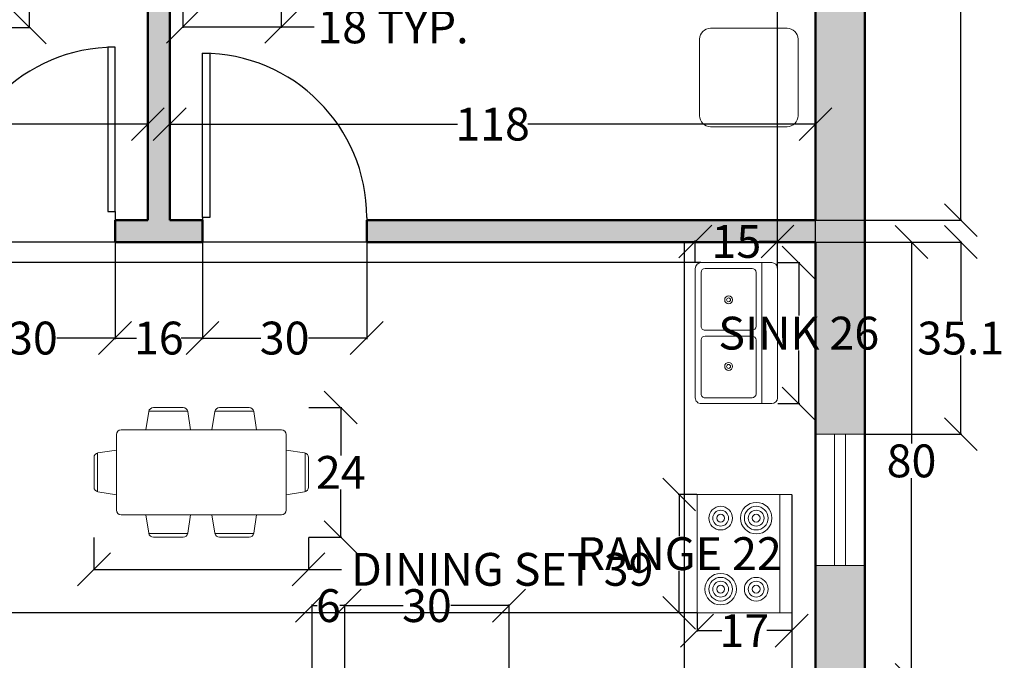
# Model space of a CAD drawing. Units: inches. Extents: x -29 to 284, y -310 to 51.
# Tile 3 of 4: x 105 to 284, y -180 to -63. Entities that reach past the tile are written whole.
import ezdxf

# ---------------------------------------------------------------- set-up
doc = ezdxf.new("R2010")
doc.units = ezdxf.units.IN
doc.header["$MEASUREMENT"] = 0
for name, color, linetype, lineweight in [('A-ANNO-DIMS', 2, 'Continuous', 18), ('A-DOOR', 3, 'Continuous', 25), ('A-EQPM', 8, 'Continuous', 18), ('A-FLOR-CASE', 9, 'Continuous', 25), ('A-FLOR-FIXT', 9, 'Continuous', 18), ('A-FURN', 8, 'Continuous', 18), ('A-GLAZ', 4, 'Continuous', 18), ('A-WALL', 7, 'Continuous', 50)]:
    doc.layers.add(name, color=color, linetype=linetype, lineweight=lineweight)
doc.layers.add('A-WALL-PATT', color=18, linetype='Continuous', lineweight=13, true_color=0x000000)
doc.styles.get("Standard").update_dxf_attribs({"font": 'arial.ttf'})
doc.dimstyles.get("Standard").update_dxf_attribs({"dimtxt": 6, "dimasz": 6, "dimexe": 0.18, "dimexo": 0.0625, "dimgap": 0.09, "dimtad": 0, "dimtih": 1, "dimtoh": 1, "dimdec": 0, "dimzin": 0, "dimdsep": 46, "dimlunit": 4, "dimtxsty": 'Standard', "dimblk": 'OBLIQUE', "dimcen": 0.09, "dimadec": 0, "dimazin": 0, "dimtfac": 1, "dimtdec": 0, "dimtofl": 0, "dimtmove": 0, "dimatfit": 3, "dimldrblk": 'OBLIQUE', "dimfxl": 1, "dimtolj": 1, "dimtzin": 0, "dimarcsym": 0})

# ---------------------------------------------------------------- blocks, each defined once
blk = doc.blocks.new('Range-Oven - 30 in top')
blk.add_line((0, -3), (30, -3))
blk.add_lwpolyline([(0, -24), (0, 0), (30, 0), (30, -24)], close=True)
for centre, radius in [((6, -9), 4), ((6, -9), 3), ((6, -9), 2), ((24, -9), 3), ((24, -9), 2), ((6, -9), 1), ((24, -9), 1), ((24, -18), 4), ((6, -18), 3), ((6, -18), 2), ((6, -18), 1), ((24, -18), 3), ((24, -18), 2), ((24, -18), 1)]:
    blk.add_circle(centre, radius)
blk = doc.blocks.new('Sink-double - 36 in top')
for p, q in [((-18, -4), (18, -4)), ((-0.75, -18.5), (-0.75, -6.5)), ((0.75, -6.5), (0.75, -18.5))]:
    blk.add_line(p, q)
for points in [[(-16.5, 0), (16.5, 0)], [(-18, -19.5), (-18, -1.5)], [(18, -1.5), (18, -19.5)], [(-16.5, -18.5), (-16.5, -6.5)], [(-15.5, -5.5), (-1.75, -5.5)], [(1.75, -5.5), (15.5, -5.5)], [(16.5, -6.5), (16.5, -18.5)], [(-1.75, -19.5), (-15.5, -19.5)], [(15.5, -19.5), (1.75, -19.5)], [(16.5, -21), (-16.5, -21)]]:
    blk.add_lwpolyline(points)
for centre, radius in [((-8.5, -12.5), 1), ((-8.5, -12.5), 0.5), ((8.5, -12.5), 1), ((8.5, -12.5), 0.5)]:
    blk.add_circle(centre, radius)
for centre, radius, start, end in [((-16.5, -1.5), 1.5, 90, 180), ((16.5, -1.5), 1.5, 0, 90), ((-15.5, -6.5), 1, 90, 180), ((-1.75, -6.5), 1, 0, 90), ((1.75, -6.5), 1, 90, 180), ((15.5, -6.5), 1, 0, 90), ((-16.5, -19.5), 1.5, 180, 270), ((-15.5, -18.5), 1, 180, 270), ((-1.75, -18.5), 1, 270, 0), ((1.75, -18.5), 1, 180, 270), ((15.5, -18.5), 1, 270, 0), ((16.5, -19.5), 1.5, 270, 0)]:
    blk.add_arc(centre, radius, start, end)
blk = doc.blocks.new('Dining Set - 36 x 72 in.')
for p, q in [((-22.26, 25.81), (-23.48, 18)), ((-22.23, 26), (-5.76, 26)), ((-20.29, 27.5), (-7.71, 27.5)), ((-4.52, 18), (-5.74, 25.81)), ((5.74, 25.81), (4.52, 18)), ((5.77, 26), (22.24, 26)), ((7.71, 27.5), (20.29, 27.5)), ((23.48, 18), (22.26, 25.81)), ((34, 18), (-34, 18)), ((-36, 16), (-36, -16)), ((36, -16), (36, 16)), ((-43.81, 8.26), (-36, 9.48)), ((43.81, 8.26), (36, 9.48)), ((-45.5, 6.29), (-45.5, -6.29)), ((-44, 8.23), (-44, -8.24)), ((44, 8.23), (44, -8.24)), ((45.5, 6.29), (45.5, -6.29)), ((-36, -9.48), (-43.81, -8.26)), ((36, -9.48), (43.81, -8.26)), ((-34, -18), (34, -18)), ((-22.26, -25.81), (-23.48, -18)), ((-4.52, -18), (-5.74, -25.81)), ((5.74, -25.81), (4.52, -18)), ((23.48, -18), (22.26, -25.81)), ((-22.23, -26), (-5.76, -26)), ((-20.29, -27.5), (-7.71, -27.5)), ((5.77, -26), (22.24, -26)), ((7.71, -27.5), (20.29, -27.5))]:
    blk.add_line(p, q)
for centre, start, end in [((-20.29, 25.5), 90, 171.1198), ((-7.71, 25.5), 8.881, 90), ((7.71, 25.5), 90, 171.1198), ((20.29, 25.5), 8.881, 90), ((-34, 16), 90, 180), ((34, 16), 0, 90), ((-43.5, 6.29), 98.8806, 180), ((43.5, 6.29), 0, 81.1194), ((-43.5, -6.29), 180, 261.1194), ((43.5, -6.29), 278.8806, 0), ((-34, -16), 180, 270), ((34, -16), 270, 0), ((-20.29, -25.5), 188.8802, 270), ((-7.71, -25.5), 270, 351.1191), ((7.71, -25.5), 188.8802, 270), ((20.29, -25.5), 270, 351.1191)]:
    blk.add_arc(centre, 2, start, end)
blk = doc.blocks.new('*U14')
for p, q in [((0, 0), (0, -6)), ((-40, 0), (-40, -6))]:
    blk.add_line(p, q)
blk.add_lwpolyline([(0, 0), (0, 40), (-1.75, 40), (-1.75, 0)], close=True)
blk.add_arc((0, 0), 40, 90, 180)
blk = doc.blocks.new('*U10')
for p, q in [((0, 0), (0, -6)), ((40, 0), (40, -6))]:
    blk.add_line(p, q)
blk.add_lwpolyline([(0, 0), (0, 40), (1.75, 40), (1.75, 0)], close=True)
blk.add_arc((0, 0), 40, 0, 90)
blk = doc.blocks.new('WIN-24IN')
for p, q in [((3.5, 24), (3.5, 0)), ((5.5, 24), (5.5, 0))]:
    blk.add_line(p, q)
for points in [[(0, 24), (9, 24)], [(9, 0), (0, 0)]]:
    blk.add_lwpolyline(points)
blk = doc.blocks.new('NIGHTSTAND-18IN')
blk.add_lwpolyline([(0, 2), (0, 16, -0.414214), (2, 18), (16, 18, -0.414214), (18, 16), (18, 2, -0.414214), (16, 0), (2, 0, -0.414214)], format="xyb", close=True)
blk = doc.blocks.new('_Oblique')
at = {"color": 0, "linetype": 'ByBlock', "lineweight": -2}
blk.add_line((-0.5, -0.5), (0.5, 0.5), dxfattribs=at)
blk = doc.blocks.new('*D26')
at = {"layer": 'A-ANNO-DIMS', "color": 0, "lineweight": -2, "transparency": 16777216}
for p, q in [((94.44, -4.36), (106.56, -4.36)), ((106.38, -4.36), (106.38, -31.2)), ((106.38, -64.36), (106.38, -37.51)), ((94.44, -64.36), (106.56, -64.36))]:
    blk.add_line(p, q, dxfattribs=at)
at = {"layer": 'Defpoints', "color": 0, "transparency": 16777216}
for p in [(94.38, -4.36), (106.38, -4.36), (94.38, -64.36)]:
    blk.add_point(p, dxfattribs=at)
at = {"layer": 'A-ANNO-DIMS', "color": 0, "lineweight": -2, "transparency": 16777216, "xscale": 6, "yscale": 6, "zscale": 6}
for p, rotation in [((106.38, -4.36), 90), ((106.38, -64.36), 270)]:
    blk.add_blockref('_Oblique', p, dxfattribs=dict(at, rotation=rotation))
at = {"layer": 'A-ANNO-DIMS', "color": 0, "transparency": 16777216, "insert": (106.38, -34.36), "char_height": 6, "attachment_point": 5}
blk.add_mtext('\\A1;60 TYP.', dxfattribs=at)
blk = doc.blocks.new('*D32')
at = {"layer": 'A-ANNO-DIMS', "color": 0, "lineweight": -2, "transparency": 16777216}
for p, q in [((134.37, -53.5), (134.37, -64.42)), ((152.37, -53.5), (152.37, -64.42)), ((134.37, -64.24), (152.37, -64.24)), ((152.37, -64.24), (158.37, -64.24))]:
    blk.add_line(p, q, dxfattribs=at)
at = {"layer": 'Defpoints', "color": 0, "transparency": 16777216}
for p in [(134.37, -53.44), (152.37, -53.44), (152.37, -64.24)]:
    blk.add_point(p, dxfattribs=at)
at = {"layer": 'A-ANNO-DIMS', "color": 0, "lineweight": -2, "transparency": 16777216, "xscale": 6, "yscale": 6, "zscale": 6, "rotation": 180}
blk.add_blockref('_Oblique', (134.37, -64.24), dxfattribs=at)
at = {"layer": 'A-ANNO-DIMS', "color": 0, "lineweight": -2, "transparency": 16777216, "xscale": 6, "yscale": 6, "zscale": 6}
blk.add_blockref('_Oblique', (152.37, -64.24), dxfattribs=at)
at = {"layer": 'A-ANNO-DIMS', "color": 0, "transparency": 16777216, "insert": (172.78, -64.24), "char_height": 6, "attachment_point": 5}
blk.add_mtext('\\A1;18 TYP.', dxfattribs=at)
blk = doc.blocks.new('*D33')
at = {"layer": 'A-ANNO-DIMS', "color": 0, "lineweight": -2, "transparency": 16777216}
for p, q in [((228.27, -149.7), (224.9, -149.7)), ((225.08, -149.7), (225.08, -157.32)), ((225.08, -171.33), (225.08, -163.71)), ((228.27, -171.33), (224.9, -171.33))]:
    blk.add_line(p, q, dxfattribs=at)
at = {"layer": 'Defpoints', "color": 0, "transparency": 16777216}
for p in [(228.33, -149.7), (225.08, -171.33), (228.33, -171.33)]:
    blk.add_point(p, dxfattribs=at)
at = {"layer": 'A-ANNO-DIMS', "color": 0, "lineweight": -2, "transparency": 16777216, "xscale": 6, "yscale": 6, "zscale": 6}
for p, rotation in [((225.08, -149.7), 90), ((225.08, -171.33), 270)]:
    blk.add_blockref('_Oblique', p, dxfattribs=dict(at, rotation=rotation))
at = {"layer": 'A-ANNO-DIMS', "color": 0, "transparency": 16777216, "insert": (225.08, -160.51), "char_height": 6, "attachment_point": 5}
blk.add_mtext('\\A1;RANGE 22', dxfattribs=at)
blk = doc.blocks.new('*D34')
at = {"layer": 'A-ANNO-DIMS', "color": 0, "lineweight": -2, "transparency": 16777216}
for p, q in [((228.33, -171.39), (228.33, -174.76)), ((245.64, -171.39), (245.64, -174.76)), ((228.33, -174.58), (232.88, -174.58)), ((245.64, -174.58), (241.09, -174.58))]:
    blk.add_line(p, q, dxfattribs=at)
at = {"layer": 'Defpoints', "color": 0, "transparency": 16777216}
for p in [(228.33, -171.33), (245.64, -171.33), (245.64, -174.58)]:
    blk.add_point(p, dxfattribs=at)
at = {"layer": 'A-ANNO-DIMS', "color": 0, "lineweight": -2, "transparency": 16777216, "xscale": 6, "yscale": 6, "zscale": 6, "rotation": 180}
blk.add_blockref('_Oblique', (228.33, -174.58), dxfattribs=at)
at = {"layer": 'A-ANNO-DIMS', "color": 0, "lineweight": -2, "transparency": 16777216, "xscale": 6, "yscale": 6, "zscale": 6}
blk.add_blockref('_Oblique', (245.64, -174.58), dxfattribs=at)
at = {"layer": 'A-ANNO-DIMS', "color": 0, "transparency": 16777216, "insert": (236.98, -174.58), "char_height": 6, "attachment_point": 5}
blk.add_mtext('\\A1;17', dxfattribs=at)
blk = doc.blocks.new('*D35')
at = {"layer": 'A-ANNO-DIMS', "color": 0, "lineweight": -2, "transparency": 16777216}
for p, q in [((243.12, -107.32), (247.1, -107.32)), ((246.92, -107.32), (246.92, -117.01)), ((246.92, -133.1), (246.92, -123.4)), ((243.12, -133.1), (247.1, -133.1))]:
    blk.add_line(p, q, dxfattribs=at)
at = {"layer": 'Defpoints', "color": 0, "transparency": 16777216}
for p in [(243.05, -107.32), (243.05, -133.1), (246.92, -133.1)]:
    blk.add_point(p, dxfattribs=at)
at = {"layer": 'A-ANNO-DIMS', "color": 0, "lineweight": -2, "transparency": 16777216, "xscale": 6, "yscale": 6, "zscale": 6}
for p, rotation in [((246.92, -107.32), 90), ((246.92, -133.1), 270)]:
    blk.add_blockref('_Oblique', p, dxfattribs=dict(at, rotation=rotation))
at = {"layer": 'A-ANNO-DIMS', "color": 0, "transparency": 16777216, "insert": (246.92, -120.21), "char_height": 6, "attachment_point": 5}
blk.add_mtext('\\A1;SINK 26', dxfattribs=at)
blk = doc.blocks.new('*D36')
at = {"layer": 'A-ANNO-DIMS', "color": 0, "lineweight": -2, "transparency": 16777216}
for p, q in [((228.01, -107.25), (228.01, -103.27)), ((228.01, -103.45), (231.41, -103.45)), ((243.05, -103.45), (239.66, -103.45)), ((243.05, -107.25), (243.05, -103.27))]:
    blk.add_line(p, q, dxfattribs=at)
at = {"layer": 'Defpoints', "color": 0, "transparency": 16777216}
for p in [(243.05, -103.45), (228.01, -107.32), (243.05, -107.32)]:
    blk.add_point(p, dxfattribs=at)
at = {"layer": 'A-ANNO-DIMS', "color": 0, "lineweight": -2, "transparency": 16777216, "xscale": 6, "yscale": 6, "zscale": 6, "rotation": 180}
blk.add_blockref('_Oblique', (228.01, -103.45), dxfattribs=at)
at = {"layer": 'A-ANNO-DIMS', "color": 0, "lineweight": -2, "transparency": 16777216, "xscale": 6, "yscale": 6, "zscale": 6}
blk.add_blockref('_Oblique', (243.05, -103.45), dxfattribs=at)
at = {"layer": 'A-ANNO-DIMS', "color": 0, "transparency": 16777216, "insert": (235.53, -103.45), "char_height": 6, "attachment_point": 5}
blk.add_mtext('\\A1;15', dxfattribs=at)
blk = doc.blocks.new('*D37')
at = {"layer": 'A-ANNO-DIMS', "color": 0, "lineweight": -2, "transparency": 16777216}
for p, q in [((118.14, -157.57), (118.14, -163.56)), ((157.35, -157.57), (157.35, -163.56)), ((118.14, -163.38), (157.35, -163.38)), ((157.35, -163.38), (163.35, -163.38))]:
    blk.add_line(p, q, dxfattribs=at)
at = {"layer": 'Defpoints', "color": 0, "transparency": 16777216}
for p in [(118.14, -157.5), (157.35, -157.5), (157.35, -163.38)]:
    blk.add_point(p, dxfattribs=at)
at = {"layer": 'A-ANNO-DIMS', "color": 0, "lineweight": -2, "transparency": 16777216, "xscale": 6, "yscale": 6, "zscale": 6, "rotation": 180}
blk.add_blockref('_Oblique', (118.14, -163.38), dxfattribs=at)
at = {"layer": 'A-ANNO-DIMS', "color": 0, "lineweight": -2, "transparency": 16777216, "xscale": 6, "yscale": 6, "zscale": 6}
blk.add_blockref('_Oblique', (157.35, -163.38), dxfattribs=at)
at = {"layer": 'A-ANNO-DIMS', "color": 0, "transparency": 16777216, "insert": (192.74, -163.38), "char_height": 6, "attachment_point": 5}
blk.add_mtext('\\A1;DINING SET 39', dxfattribs=at)
blk = doc.blocks.new('*D38')
at = {"layer": 'A-ANNO-DIMS', "color": 0, "lineweight": -2, "transparency": 16777216}
for p, q in [((157.41, -133.81), (163.41, -133.81)), ((163.23, -133.81), (163.23, -142.55)), ((163.23, -157.5), (163.23, -148.76)), ((157.41, -157.5), (163.41, -157.5))]:
    blk.add_line(p, q, dxfattribs=at)
at = {"layer": 'Defpoints', "color": 0, "transparency": 16777216}
for p in [(157.35, -133.81), (163.23, -133.81), (157.35, -157.5)]:
    blk.add_point(p, dxfattribs=at)
at = {"layer": 'A-ANNO-DIMS', "color": 0, "lineweight": -2, "transparency": 16777216, "xscale": 6, "yscale": 6, "zscale": 6}
for p, rotation in [((163.23, -133.81), 90), ((163.23, -157.5), 270)]:
    blk.add_blockref('_Oblique', p, dxfattribs=dict(at, rotation=rotation))
at = {"layer": 'A-ANNO-DIMS', "color": 0, "transparency": 16777216, "insert": (163.23, -145.66), "char_height": 6, "attachment_point": 5}
blk.add_mtext('\\A1;24', dxfattribs=at)
blk = doc.blocks.new('*D51')
at = {"layer": 'A-ANNO-DIMS', "color": 0, "lineweight": -2, "transparency": 16777216}
for p, q in [((250.04, 20.44), (276.71, 20.44)), ((276.53, 20.44), (276.53, -36.41)), ((276.53, -99.56), (276.53, -42.72)), ((250.04, -99.56), (276.71, -99.56))]:
    blk.add_line(p, q, dxfattribs=at)
at = {"layer": 'Defpoints', "color": 0, "transparency": 16777216}
for p in [(249.98, 20.44), (249.98, -99.56), (276.53, -99.56)]:
    blk.add_point(p, dxfattribs=at)
at = {"layer": 'A-ANNO-DIMS', "color": 0, "lineweight": -2, "transparency": 16777216, "xscale": 6, "yscale": 6, "zscale": 6}
for p, rotation in [((276.53, 20.44), 90), ((276.53, -99.56), 270)]:
    blk.add_blockref('_Oblique', p, dxfattribs=dict(at, rotation=rotation))
at = {"layer": 'A-ANNO-DIMS', "color": 0, "transparency": 16777216, "insert": (276.53, -39.56), "char_height": 6, "attachment_point": 5}
blk.add_mtext('\\A1;120', dxfattribs=at)
blk = doc.blocks.new('*D52')
at = {"layer": 'A-ANNO-DIMS', "color": 0, "lineweight": -2, "transparency": 16777216}
for p, q in [((9.98, -99.5), (9.98, -81.83)), ((9.98, -82.01), (62.54, -82.01)), ((127.98, -82.01), (75.42, -82.01)), ((127.98, -99.5), (127.98, -81.83))]:
    blk.add_line(p, q, dxfattribs=at)
at = {"layer": 'Defpoints', "color": 0, "transparency": 16777216}
for p in [(127.98, -82.01), (9.98, -99.56), (127.98, -99.56)]:
    blk.add_point(p, dxfattribs=at)
at = {"layer": 'A-ANNO-DIMS', "color": 0, "lineweight": -2, "transparency": 16777216, "xscale": 6, "yscale": 6, "zscale": 6, "rotation": 180}
blk.add_blockref('_Oblique', (9.98, -82.01), dxfattribs=at)
at = {"layer": 'A-ANNO-DIMS', "color": 0, "lineweight": -2, "transparency": 16777216, "xscale": 6, "yscale": 6, "zscale": 6}
blk.add_blockref('_Oblique', (127.98, -82.01), dxfattribs=at)
at = {"layer": 'A-ANNO-DIMS', "color": 0, "transparency": 16777216, "insert": (68.98, -82.01), "char_height": 6, "attachment_point": 5}
blk.add_mtext('\\A1;118', dxfattribs=at)
blk = doc.blocks.new('*D53')
at = {"layer": 'A-ANNO-DIMS', "color": 0, "lineweight": -2, "transparency": 16777216}
for p, q in [((131.98, -99.5), (131.98, -81.83)), ((131.98, -82.01), (184.54, -82.01)), ((249.98, -82.01), (197.42, -82.01)), ((249.98, -99.5), (249.98, -81.83))]:
    blk.add_line(p, q, dxfattribs=at)
at = {"layer": 'Defpoints', "color": 0, "transparency": 16777216}
for p in [(249.98, -82.01), (131.98, -99.56), (249.98, -99.56)]:
    blk.add_point(p, dxfattribs=at)
at = {"layer": 'A-ANNO-DIMS', "color": 0, "lineweight": -2, "transparency": 16777216, "xscale": 6, "yscale": 6, "zscale": 6, "rotation": 180}
blk.add_blockref('_Oblique', (131.98, -82.01), dxfattribs=at)
at = {"layer": 'A-ANNO-DIMS', "color": 0, "lineweight": -2, "transparency": 16777216, "xscale": 6, "yscale": 6, "zscale": 6}
blk.add_blockref('_Oblique', (249.98, -82.01), dxfattribs=at)
at = {"layer": 'A-ANNO-DIMS', "color": 0, "transparency": 16777216, "insert": (190.98, -82.01), "char_height": 6, "attachment_point": 5}
blk.add_mtext('\\A1;118', dxfattribs=at)
blk = doc.blocks.new('*D55')
at = {"layer": 'A-ANNO-DIMS', "color": 0, "lineweight": -2, "transparency": 16777216}
for p, q in [((91.98, -103.63), (91.98, -121.29)), ((121.98, -103.63), (121.98, -121.29)), ((91.98, -121.11), (102.61, -121.11)), ((121.98, -121.11), (111.36, -121.11))]:
    blk.add_line(p, q, dxfattribs=at)
at = {"layer": 'Defpoints', "color": 0, "transparency": 16777216}
for p in [(91.98, -103.56), (121.98, -103.56), (91.98, -121.11)]:
    blk.add_point(p, dxfattribs=at)
at = {"layer": 'A-ANNO-DIMS', "color": 0, "lineweight": -2, "transparency": 16777216, "xscale": 6, "yscale": 6, "zscale": 6, "rotation": 180}
blk.add_blockref('_Oblique', (91.98, -121.11), dxfattribs=at)
at = {"layer": 'A-ANNO-DIMS', "color": 0, "lineweight": -2, "transparency": 16777216, "xscale": 6, "yscale": 6, "zscale": 6}
blk.add_blockref('_Oblique', (121.98, -121.11), dxfattribs=at)
at = {"layer": 'A-ANNO-DIMS', "color": 0, "transparency": 16777216, "insert": (106.98, -121.11), "char_height": 6, "attachment_point": 5}
blk.add_mtext('\\A1;30', dxfattribs=at)
blk = doc.blocks.new('*D56')
at = {"layer": 'A-ANNO-DIMS', "color": 0, "lineweight": -2, "transparency": 16777216}
for p, q in [((121.98, -103.63), (121.98, -121.29)), ((137.98, -103.63), (137.98, -121.29)), ((121.98, -121.11), (125.88, -121.11)), ((137.98, -121.11), (134.08, -121.11))]:
    blk.add_line(p, q, dxfattribs=at)
at = {"layer": 'Defpoints', "color": 0, "transparency": 16777216}
for p in [(121.98, -103.56), (137.98, -103.56), (121.98, -121.11)]:
    blk.add_point(p, dxfattribs=at)
at = {"layer": 'A-ANNO-DIMS', "color": 0, "lineweight": -2, "transparency": 16777216, "xscale": 6, "yscale": 6, "zscale": 6, "rotation": 180}
blk.add_blockref('_Oblique', (121.98, -121.11), dxfattribs=at)
at = {"layer": 'A-ANNO-DIMS', "color": 0, "lineweight": -2, "transparency": 16777216, "xscale": 6, "yscale": 6, "zscale": 6}
blk.add_blockref('_Oblique', (137.98, -121.11), dxfattribs=at)
at = {"layer": 'A-ANNO-DIMS', "color": 0, "transparency": 16777216, "insert": (129.98, -121.11), "char_height": 6, "attachment_point": 5}
blk.add_mtext('\\A1;16', dxfattribs=at)
blk = doc.blocks.new('*D57')
at = {"layer": 'A-ANNO-DIMS', "color": 0, "lineweight": -2, "transparency": 16777216}
for p, q in [((137.98, -103.63), (137.98, -121.29)), ((167.98, -103.63), (167.98, -121.29)), ((137.98, -121.11), (148.61, -121.11)), ((167.98, -121.11), (157.36, -121.11))]:
    blk.add_line(p, q, dxfattribs=at)
at = {"layer": 'Defpoints', "color": 0, "transparency": 16777216}
for p in [(137.98, -103.56), (167.98, -103.56), (137.98, -121.11)]:
    blk.add_point(p, dxfattribs=at)
at = {"layer": 'A-ANNO-DIMS', "color": 0, "lineweight": -2, "transparency": 16777216, "xscale": 6, "yscale": 6, "zscale": 6, "rotation": 180}
blk.add_blockref('_Oblique', (137.98, -121.11), dxfattribs=at)
at = {"layer": 'A-ANNO-DIMS', "color": 0, "lineweight": -2, "transparency": 16777216, "xscale": 6, "yscale": 6, "zscale": 6}
blk.add_blockref('_Oblique', (167.98, -121.11), dxfattribs=at)
at = {"layer": 'A-ANNO-DIMS', "color": 0, "transparency": 16777216, "insert": (152.98, -121.11), "char_height": 6, "attachment_point": 5}
blk.add_mtext('\\A1;30', dxfattribs=at)
blk = doc.blocks.new('*D64')
at = {"layer": 'A-ANNO-DIMS', "color": 0, "lineweight": -2, "transparency": 16777216}
for p, q in [((250.04, -103.56), (276.71, -103.56)), ((276.53, -103.56), (276.53, -117.96)), ((276.53, -138.66), (276.53, -124.27)), ((259.04, -138.66), (276.71, -138.66))]:
    blk.add_line(p, q, dxfattribs=at)
at = {"layer": 'Defpoints', "color": 0, "transparency": 16777216}
for p in [(249.98, -103.56), (276.53, -103.56), (258.98, -138.66)]:
    blk.add_point(p, dxfattribs=at)
at = {"layer": 'A-ANNO-DIMS', "color": 0, "lineweight": -2, "transparency": 16777216, "xscale": 6, "yscale": 6, "zscale": 6}
for p, rotation in [((276.53, -103.56), 90), ((276.53, -138.66), 270)]:
    blk.add_blockref('_Oblique', p, dxfattribs=dict(at, rotation=rotation))
at = {"layer": 'A-ANNO-DIMS', "color": 0, "transparency": 16777216, "insert": (276.53, -121.11), "char_height": 6, "attachment_point": 5}
blk.add_mtext('\\A1;35.1', dxfattribs=at)
blk = doc.blocks.new('*D65')
at = {"layer": 'A-ANNO-DIMS', "color": 0, "lineweight": -2, "transparency": 16777216}
for p, q in [((250.04, -103.56), (267.71, -103.56)), ((267.53, -103.56), (267.53, -140.41)), ((267.53, -183.56), (267.53, -146.72)), ((250.04, -183.56), (267.71, -183.56))]:
    blk.add_line(p, q, dxfattribs=at)
at = {"layer": 'Defpoints', "color": 0, "transparency": 16777216}
for p in [(249.98, -103.56), (249.98, -183.56), (267.53, -183.56)]:
    blk.add_point(p, dxfattribs=at)
at = {"layer": 'A-ANNO-DIMS', "color": 0, "lineweight": -2, "transparency": 16777216, "xscale": 6, "yscale": 6, "zscale": 6}
for p, rotation in [((267.53, -103.56), 90), ((267.53, -183.56), 270)]:
    blk.add_blockref('_Oblique', p, dxfattribs=dict(at, rotation=rotation))
at = {"layer": 'A-ANNO-DIMS', "color": 0, "transparency": 16777216, "insert": (267.53, -143.56), "char_height": 6, "attachment_point": 5}
blk.add_mtext('\\A1;80', dxfattribs=at)
blk = doc.blocks.new('*D66')
at = {"layer": 'A-ANNO-DIMS', "color": 0, "lineweight": -2, "transparency": 16777216}
for p, q in [((-16.57, -103.56), (-16.57, -97.56)), ((-16.57, -97.56), (-10.57, -97.56)), ((225.92, -103.56), (-16.75, -103.56)), ((-16.57, -107.32), (-16.57, -103.56)), ((229.03, -107.32), (-16.75, -107.32))]:
    blk.add_line(p, q, dxfattribs=at)
at = {"layer": 'Defpoints', "color": 0, "transparency": 16777216}
for p in [(-16.57, -103.56), (225.98, -103.56), (229.09, -107.32)]:
    blk.add_point(p, dxfattribs=at)
at = {"layer": 'A-ANNO-DIMS', "color": 0, "lineweight": -2, "transparency": 16777216, "xscale": 6, "yscale": 6, "zscale": 6}
for p, rotation in [((-16.57, -103.56), 90), ((-16.57, -107.32), 270)]:
    blk.add_blockref('_Oblique', p, dxfattribs=dict(at, rotation=rotation))
at = {"layer": 'A-ANNO-DIMS', "color": 0, "transparency": 16777216, "insert": (-0.39, -97.56), "char_height": 6, "attachment_point": 5}
blk.add_mtext('\\A1;3.752', dxfattribs=at)
blk = doc.blocks.new('*D67')
at = {"layer": 'A-ANNO-DIMS', "color": 0, "lineweight": -2, "transparency": 16777216}
for p, q in [((228.27, -171.33), (-16.75, -171.33)), ((-16.57, -171.33), (-16.57, -174.29)), ((-16.57, -183.56), (-16.57, -180.6)), ((225.92, -183.56), (-16.75, -183.56))]:
    blk.add_line(p, q, dxfattribs=at)
at = {"layer": 'Defpoints', "color": 0, "transparency": 16777216}
for p in [(228.33, -171.33), (-16.57, -183.56), (225.98, -183.56)]:
    blk.add_point(p, dxfattribs=at)
at = {"layer": 'A-ANNO-DIMS', "color": 0, "lineweight": -2, "transparency": 16777216, "xscale": 6, "yscale": 6, "zscale": 6}
for p, rotation in [((-16.57, -171.33), 90), ((-16.57, -183.56), 270)]:
    blk.add_blockref('_Oblique', p, dxfattribs=dict(at, rotation=rotation))
at = {"layer": 'A-ANNO-DIMS', "color": 0, "transparency": 16777216, "insert": (-16.57, -177.45), "char_height": 6, "attachment_point": 5}
blk.add_mtext('\\A1;12.233', dxfattribs=at)
blk = doc.blocks.new('*D68')
at = {"layer": 'A-ANNO-DIMS', "color": 0, "lineweight": -2, "transparency": 16777216}
for p, q in [((243.05, -108.33), (243.05, 47.17)), ((243.05, 46.99), (249.98, 46.99)), ((249.98, -103.5), (249.98, 47.17)), ((249.98, 46.99), (255.98, 46.99))]:
    blk.add_line(p, q, dxfattribs=at)
at = {"layer": 'Defpoints', "color": 0, "transparency": 16777216}
for p in [(249.98, 46.99), (249.98, -103.56), (243.05, -108.39)]:
    blk.add_point(p, dxfattribs=at)
at = {"layer": 'A-ANNO-DIMS', "color": 0, "lineweight": -2, "transparency": 16777216, "xscale": 6, "yscale": 6, "zscale": 6, "rotation": 180}
blk.add_blockref('_Oblique', (243.05, 46.99), dxfattribs=at)
at = {"layer": 'A-ANNO-DIMS', "color": 0, "lineweight": -2, "transparency": 16777216, "xscale": 6, "yscale": 6, "zscale": 6}
blk.add_blockref('_Oblique', (249.98, 46.99), dxfattribs=at)
at = {"layer": 'A-ANNO-DIMS', "color": 0, "transparency": 16777216, "insert": (266.21, 46.99), "char_height": 6, "attachment_point": 5}
blk.add_mtext('\\A1;6.927', dxfattribs=at)
blk = doc.blocks.new('*D69')
at = {"layer": 'A-ANNO-DIMS', "color": 0, "lineweight": -2, "transparency": 16777216}
for p, q in [((249.98, -138.72), (249.98, -306.29)), ((245.64, -149.76), (245.64, -306.29)), ((245.64, -306.11), (249.98, -306.11)), ((249.98, -306.11), (255.98, -306.11))]:
    blk.add_line(p, q, dxfattribs=at)
at = {"layer": 'Defpoints', "color": 0, "transparency": 16777216}
for p in [(249.98, -138.66), (245.64, -149.7), (249.98, -306.11)]:
    blk.add_point(p, dxfattribs=at)
at = {"layer": 'A-ANNO-DIMS', "color": 0, "lineweight": -2, "transparency": 16777216, "xscale": 6, "yscale": 6, "zscale": 6, "rotation": 180}
blk.add_blockref('_Oblique', (245.64, -306.11), dxfattribs=at)
at = {"layer": 'A-ANNO-DIMS', "color": 0, "lineweight": -2, "transparency": 16777216, "xscale": 6, "yscale": 6, "zscale": 6}
blk.add_blockref('_Oblique', (249.98, -306.11), dxfattribs=at)
at = {"layer": 'A-ANNO-DIMS', "color": 0, "transparency": 16777216, "insert": (263.97, -306.11), "char_height": 6, "attachment_point": 5}
blk.add_mtext('\\A1;4.34', dxfattribs=at)
blk = doc.blocks.new('*D73')
at = {"layer": 'A-ANNO-DIMS', "color": 0, "lineweight": -2, "transparency": 16777216}
for p, q in [((157.98, -187.5), (157.98, -169.83)), ((157.98, -170.01), (158.91, -170.01)), ((163.98, -170.01), (163.05, -170.01)), ((163.98, -187.5), (163.98, -169.83))]:
    blk.add_line(p, q, dxfattribs=at)
at = {"layer": 'Defpoints', "color": 0, "transparency": 16777216}
for p in [(163.98, -170.01), (157.98, -187.56), (163.98, -187.56)]:
    blk.add_point(p, dxfattribs=at)
at = {"layer": 'A-ANNO-DIMS', "color": 0, "lineweight": -2, "transparency": 16777216, "xscale": 6, "yscale": 6, "zscale": 6, "rotation": 180}
blk.add_blockref('_Oblique', (157.98, -170.01), dxfattribs=at)
at = {"layer": 'A-ANNO-DIMS', "color": 0, "lineweight": -2, "transparency": 16777216, "xscale": 6, "yscale": 6, "zscale": 6}
blk.add_blockref('_Oblique', (163.98, -170.01), dxfattribs=at)
at = {"layer": 'A-ANNO-DIMS', "color": 0, "transparency": 16777216, "insert": (160.98, -170.01), "char_height": 6, "attachment_point": 5}
blk.add_mtext('\\A1;6', dxfattribs=at)
blk = doc.blocks.new('*D74')
at = {"layer": 'A-ANNO-DIMS', "color": 0, "lineweight": -2, "transparency": 16777216}
for p, q in [((163.98, -187.5), (163.98, -169.83)), ((163.98, -170.01), (174.61, -170.01)), ((193.98, -170.01), (183.36, -170.01)), ((193.98, -187.5), (193.98, -169.83))]:
    blk.add_line(p, q, dxfattribs=at)
at = {"layer": 'Defpoints', "color": 0, "transparency": 16777216}
for p in [(193.98, -170.01), (163.98, -187.56), (193.98, -187.56)]:
    blk.add_point(p, dxfattribs=at)
at = {"layer": 'A-ANNO-DIMS', "color": 0, "lineweight": -2, "transparency": 16777216, "xscale": 6, "yscale": 6, "zscale": 6, "rotation": 180}
blk.add_blockref('_Oblique', (163.98, -170.01), dxfattribs=at)
at = {"layer": 'A-ANNO-DIMS', "color": 0, "lineweight": -2, "transparency": 16777216, "xscale": 6, "yscale": 6, "zscale": 6}
blk.add_blockref('_Oblique', (193.98, -170.01), dxfattribs=at)
at = {"layer": 'A-ANNO-DIMS', "color": 0, "transparency": 16777216, "insert": (178.98, -170.01), "char_height": 6, "attachment_point": 5}
blk.add_mtext('\\A1;30', dxfattribs=at)

msp = doc.modelspace()

# ---------------------------------------------------------------- hatches: boundary and pattern name
at = {"layer": 'A-WALL-PATT'}
h = msp.add_hatch(color=256, dxfattribs=at)
h.dxf.hatch_style = 1
h.paths.add_polyline_path([(172.6409, 20.4365), (172.6409, 29.4365), (82.1984, 29.4365), (82.1984, 20.4365), (127.9809, 20.4365), (127.9809, -99.5635), (121.9809, -99.5635), (121.9809, -103.5635), (127.9809, -103.5635), (137.9809, -103.5635), (137.9809, -99.5635), (131.9809, -99.5635), (131.9809, 20.4365)])
h = msp.add_hatch(color=256, dxfattribs=at)
h.dxf.hatch_style = 1
h.paths.add_polyline_path([(249.9809, 20.4365), (249.9809, -99.5635), (167.9809, -99.5635), (167.9809, -103.5635), (249.9809, -103.5635), (249.9809, -138.6614), (258.9809, -138.6614), (258.9809, 29.4365), (220.6409, 29.4365), (220.6409, 20.4365)])
h = msp.add_hatch(color=256, dxfattribs=at)
h.dxf.hatch_style = 1
h.paths.add_polyline_path([(258.9809, -162.6614), (249.9809, -162.6614), (249.9809, -183.5635), (193.9809, -183.5635), (193.9809, -187.5635), (249.9809, -187.5635), (249.9809, -279.5635), (227.3376, -279.5635), (227.3376, -288.5635), (258.9809, -288.5635)])

# ---------------------------------------------------------------- linework, layer by layer
at = {"layer": 'A-FLOR-CASE'}
msp.add_line((225.9809, -103.5635), (225.9809, -183.5635), dxfattribs=at)
at = {"layer": 'A-WALL'}
for p, q in [((127.9809, -99.5635), (127.9809, 20.4365)), ((131.9809, -99.5635), (131.9809, 20.4365)), ((249.9809, 20.4365), (249.9809, -99.5635)), ((121.9809, -99.5635), (121.9809, -103.5635)), ((121.9809, -99.5635), (127.9809, -99.5635)), ((131.9809, -99.5635), (137.9809, -99.5635)), ((137.9809, -99.5635), (137.9809, -103.5635)), ((167.9809, -99.5635), (167.9809, -103.5635)), ((167.9809, -99.5635), (249.9809, -99.5635)), ((121.9809, -103.5635), (127.9809, -103.5635)), ((127.9809, -103.5635), (137.9809, -103.5635)), ((167.9809, -103.5635), (249.9809, -103.5635)), ((249.9809, -103.5635), (249.9809, -183.5635))]:
    msp.add_line(p, q, dxfattribs=at)
msp.add_lwpolyline([(99.9809, -288.5635), (0.9809, -288.5635), (0.9809, 29.4365), (258.9809, 29.4365), (258.9809, -288.5635), (135.9809, -288.5635)], dxfattribs=at)

# ---------------------------------------------------------------- block references
at = {"layer": 'A-DOOR', "xscale": 0.75, "yscale": 0.75, "zscale": 0.75}
for name, p in [('*U14', (121.9809, -97.9623)), ('*U10', (137.9809, -99.0635))]:
    msp.add_blockref(name, p, dxfattribs=at)
at = {"layer": 'A-EQPM', "xscale": 0.7211102624887981, "yscale": 0.7211102624887981, "zscale": 0.7211102624887981, "rotation": 270}
msp.add_blockref('Range-Oven - 30 in top', (245.6365, -149.6968), dxfattribs=at)
at = {"layer": 'A-FLOR-FIXT', "xscale": 0.7161952055979305, "yscale": 0.7161952055979305, "zscale": 0.7161952055979305, "rotation": 270}
msp.add_blockref('Sink-double - 36 in top', (243.054, -120.2072), dxfattribs=at)
at = {"layer": 'A-FURN', "rotation": 180}
msp.add_blockref('NIGHTSTAND-18IN', (246.7929, -64.4778), dxfattribs=at)
at = {"layer": 'A-FURN', "xscale": 0.430826044735534, "yscale": 0.430826044735534, "zscale": 0.430826044735534}
msp.add_blockref('Dining Set - 36 x 72 in.', (137.7445, -145.6565), dxfattribs=at)
at = {"layer": 'A-GLAZ'}
msp.add_blockref('WIN-24IN', (249.981, -162.661), dxfattribs=at)

# ---------------------------------------------------------------- dimensions: what is measured, and where the dimension line sits
at = {"layer": 'A-ANNO-DIMS'}
for base, p1, p2, override, picture, middle in [((249.9809, 46.9865), (243.054, -108.39), (249.9809, -103.5635), {"dimdec": 3, "dimlfac": 1, "dimrnd": 0, "dimzin": 0, "dimdsep": 46, "dimlunit": 2}, '*D68', (266.2108, 46.9865)), ((127.9809, -82.0135), (9.9809, -99.5635), (127.9809, -99.5635), {"dimdec": 0, "dimlfac": 1, "dimrnd": 0, "dimzin": 0, "dimdsep": 46, "dimlunit": 2}, '*D52', (68.9809, -82.0135)), ((249.9809, -82.0135), (131.9809, -99.5635), (249.9809, -99.5635), {"dimdec": 0, "dimlfac": 1, "dimrnd": 0, "dimzin": 0, "dimdsep": 46, "dimlunit": 2}, '*D53', (190.9809, -82.0135)), ((243.054, -103.4482), (228.0139, -107.3157), (243.054, -107.3157), {"dimdec": 0, "dimlfac": 1, "dimrnd": 0, "dimzin": 0, "dimdsep": 46, "dimlunit": 2}, '*D36', (235.5339, -103.4482)), ((249.9809, -306.1135), (245.6365, -149.6968), (249.9809, -138.6614), {"dimdec": 2, "dimlfac": 1, "dimrnd": 0, "dimzin": 0, "dimdsep": 46, "dimlunit": 2}, '*D69', (263.972, -306.1135)), ((163.9809, -170.0135), (157.9809, -187.5635), (163.9809, -187.5635), {"dimdec": 0, "dimlfac": 1, "dimrnd": 0, "dimzin": 0, "dimdsep": 46, "dimlunit": 2}, '*D73', (160.9809, -170.0135)), ((193.9809, -170.0135), (163.9809, -187.5635), (193.9809, -187.5635), {"dimdec": 0, "dimlfac": 1, "dimrnd": 0, "dimzin": 0, "dimdsep": 46, "dimlunit": 2}, '*D74', (178.9809, -170.0135)), ((245.6365, -174.5751), (228.3299, -171.3301), (245.6365, -171.3301), {"dimdec": 0, "dimlfac": 1, "dimrnd": 0, "dimzin": 0, "dimdsep": 46, "dimlunit": 2}, '*D34', (236.9832, -174.5751))]:
    dim = msp.add_linear_dim(base=base, p1=p1, p2=p2, dimstyle='Standard', override=override, dxfattribs=at)
    dim.commit()
    dim.dimension.update_dxf_attribs({"geometry": picture, "text_midpoint": middle})
for base, p1, p2, angle, override, picture, middle in [((276.5309, -99.5635), (249.9809, 20.4365), (249.9809, -99.5635), 90, {"dimdec": 0, "dimlfac": 1, "dimrnd": 0, "dimzin": 0, "dimdsep": 46, "dimlunit": 2}, '*D51', (276.5309, -39.5635)), ((-16.5691, -103.5635), (229.0882, -107.3157), (225.9809, -103.5635), 90, {"dimdec": 3, "dimlfac": 1, "dimrnd": 0, "dimzin": 0, "dimdsep": 46, "dimlunit": 2}, '*D66', (-0.3883, -97.5635)), ((276.5309, -103.5635), (258.9809, -138.6614), (249.9809, -103.5635), 90, {"dimdec": 1, "dimlfac": 1, "dimrnd": 0, "dimzin": 0, "dimdsep": 46, "dimlunit": 2}, '*D64', (276.5309, -121.1124)), ((267.5309, -183.5635), (249.9809, -103.5635), (249.9809, -183.5635), 270, {"dimdec": 0, "dimlfac": 1, "dimrnd": 0, "dimzin": 0, "dimdsep": 46, "dimlunit": 2}, '*D65', (267.5309, -143.5635)), ((91.9809, -121.1135), (121.9809, -103.5635), (91.9809, -103.5635), 180, {"dimdec": 0, "dimlfac": 1, "dimrnd": 0, "dimzin": 0, "dimdsep": 46, "dimlunit": 2}, '*D55', (106.9809, -121.1135)), ((121.9809, -121.1135), (137.9809, -103.5635), (121.9809, -103.5635), 180, {"dimdec": 0, "dimlfac": 1, "dimrnd": 0, "dimzin": 0, "dimdsep": 46, "dimlunit": 2}, '*D56', (129.9809, -121.1135)), ((137.9809, -121.1135), (167.9809, -103.5635), (137.9809, -103.5635), 180, {"dimdec": 0, "dimlfac": 1, "dimrnd": 0, "dimzin": 0, "dimdsep": 46, "dimlunit": 2}, '*D57', (152.9809, -121.1135)), ((163.2279, -133.8088), (157.3471, -157.5042), (157.3471, -133.8088), 90, {"dimdec": 0, "dimlfac": 1, "dimrnd": 0, "dimzin": 0, "dimdsep": 46, "dimlunit": 2}, '*D38', (163.2279, -145.6565)), ((-16.5691, -183.5635), (228.3299, -171.3301), (225.9809, -183.5635), 90, {"dimdec": 3, "dimlfac": 1, "dimrnd": 0, "dimzin": 0, "dimdsep": 46, "dimlunit": 2}, '*D67', (-16.5691, -177.4468))]:
    dim = msp.add_linear_dim(base=base, p1=p1, p2=p2, angle=angle, dimstyle='Standard', override=override, dxfattribs=at)
    dim.commit()
    dim.dimension.update_dxf_attribs({"geometry": picture, "text_midpoint": middle})
for base, p1, p2, angle, text, picture, middle in [((106.3804, -4.3576), (94.3804, -64.3576), (94.3804, -4.3576), 90, '<> TYP.', '*D26', (106.3804, -34.3576)), ((246.9215, -133.0987), (243.054, -107.3157), (243.054, -133.0987), 270, 'SINK <>', '*D35', (246.9215, -120.2072)), ((225.0849, -171.3301), (228.3299, -149.6968), (228.3299, -171.3301), 270, 'RANGE <>', '*D33', (225.0849, -160.5134))]:
    dim = msp.add_linear_dim(base=base, p1=p1, p2=p2, angle=angle, text=text, dimstyle='Standard', override={"dimdec": 0, "dimlfac": 1, "dimrnd": 0, "dimzin": 0, "dimdsep": 46, "dimlunit": 2}, dxfattribs=at)
    dim.commit()
    dim.dimension.update_dxf_attribs({"geometry": picture, "text_midpoint": middle})
for base, p1, p2, text, picture, middle in [((152.3688, -64.2404), (134.3688, -53.4404), (152.3688, -53.4404), '<> TYP.', '*D32', (172.7794, -64.2404)), ((157.3471, -163.385), (118.1419, -157.5042), (157.3471, -157.5042), 'DINING SET <>', '*D37', (192.7393, -163.385))]:
    dim = msp.add_linear_dim(base=base, p1=p1, p2=p2, text=text, dimstyle='Standard', override={"dimdec": 0, "dimlfac": 1, "dimrnd": 0, "dimzin": 0, "dimdsep": 46, "dimlunit": 2}, dxfattribs=at)
    dim.commit()
    dim.dimension.update_dxf_attribs({"geometry": picture, "text_midpoint": middle})

doc.saveas('drawing.dxf')
